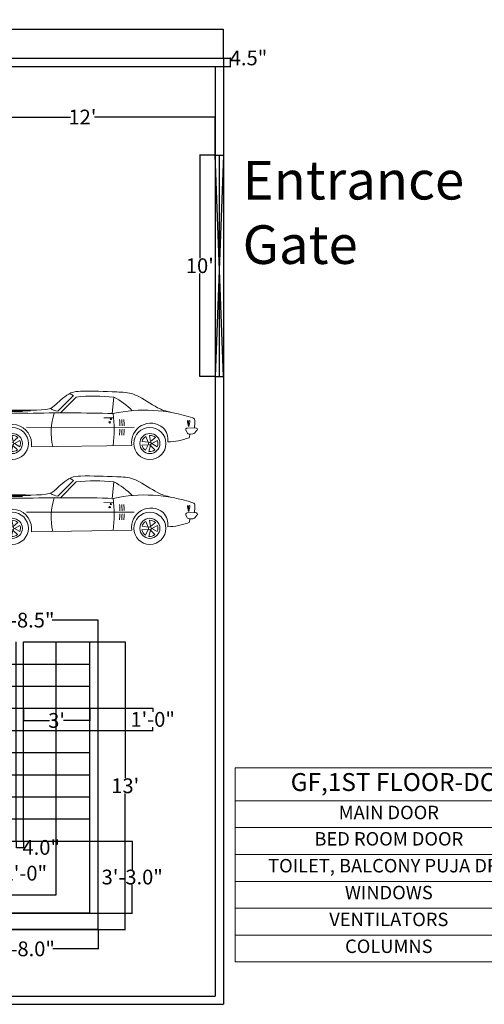
# Model space of a CAD drawing. Units: inches. Extents: x 20414 to 21627, y 49019 to 50314.
# Tile 9 of 10: x 20835 to 21087, y 49781 to 50314. Entities that reach past the tile are written whole.
import ezdxf

# ---------------------------------------------------------------- set-up
doc = ezdxf.new("R2010")
doc.units = ezdxf.units.IN
for name, color, linetype, lineweight in [('A-ANNO-DIMS', 7, 'Continuous', 18), ('A-ANNO-SCHD', 7, 'Continuous', 18), ('C-PROP', 6, 'Continuous', 25), ('C-SITE-GATE', 3, 'Continuous', 25), ('cars', 40, 'Continuous', 13), ('stairs', 4, 'Continuous', 25), ('text', 3, 'Continuous', 25), ('walls', 6, 'Continuous', 35)]:
    doc.layers.add(name, color=color, linetype=linetype, lineweight=lineweight)
doc.styles.get("Standard").update_dxf_attribs({"font": 'arial.ttf'})
doc.dimstyles.get("Standard").update_dxf_attribs({"dimtxt": 8, "dimasz": 0.18, "dimexe": 0.18, "dimexo": 0.0625, "dimgap": 0.09, "dimtad": 0, "dimtih": 1, "dimtoh": 1, "dimdec": 1, "dimzin": 0, "dimdsep": 46, "dimlunit": 3, "dimtxsty": 'Standard', "dimcen": 0.09, "dimadec": 0, "dimazin": 0, "dimtfac": 1, "dimtdec": 1, "dimtofl": 0, "dimtmove": 0, "dimatfit": 3, "dimfxl": 1, "dimtolj": 1, "dimtzin": 0, "dimarcsym": 0})

# ---------------------------------------------------------------- blocks, each defined once
blk = doc.blocks.new('*U25')
for p, q in [((1852, 1022), (2179, 1351)), ((1905, 986), (2237, 1320)), ((3032, 1318), (2995, 973)), ((1273, 1043), (872, 1041)), ((1099, 1012), (893, 1010)), ((897, 1028), (1273, 1032)), ((2822, 882), (3009, 880)), ((1185, 681), (3462, 680)), ((4581, 665), (4763, 671)), ((189, 502), (247, 503)), ((248, 455), (217, 455)), ((263, 487), (264, 471)), ((4554, 619), (4578, 571)), ((4639, 537), (4697, 540)), ((4742, 563), (4788, 619)), ((1292, 344), (1293, 267))]:
    blk.add_line(p, q)
for points in [[(897, 1014), (897, 1023, 0.269532), (893, 1030), (873, 1041, 0.575383), (867, 1037), (868, 1028, 0.269532), (872, 1022), (891, 1011, 0.575383)], [(724, 383), (854, 366), (804, 487, 0.199906)], [(880, 509), (903, 380), (1003, 465, 0.199906)], [(3628, 383), (3758, 366), (3709, 487, 0.199906)], [(3784, 509), (3808, 380), (3908, 465, 0.199906)], [(795, 196), (852, 314), (721, 305, 0.199906)], [(995, 206), (901, 297), (870, 170, 0.199906)], [(1048, 400), (932, 338), (1044, 269, 0.199906)], [(3700, 196), (3757, 314), (3626, 305, 0.199906)], [(3900, 206), (3805, 297), (3774, 170, 0.199906)], [(3952, 400), (3837, 338), (3948, 269, 0.199906)]]:
    blk.add_lwpolyline(points, format="xyb", close=True)
for points in [[(4612, 698), (4611, 811), (4584, 824)], [(4612, 698), (4611, 811), (4637, 824)], [(1293, 267), (3413, 300)]]:
    blk.add_lwpolyline(points)
for centre, radius in [((888, 339), 339), ((2944, 788), 15.7), ((3793, 339), 339), ((888, 339), 212), ((3793, 339), 212), ((888, 339), 31.7), ((3793, 339), 31.7)]:
    blk.add_circle(centre, radius)
for centre, radius, start, end in [((2911, 2669), 1508, 237.6103, 240.9785), ((2628, -2413), 3754, 83.8163, 95.9705), ((2426, 99), 1362, 43.2748, 63.5665), ((1861, 1282), 261, 230.424, 268.0085), ((3687, -2156), 3200, 71.5283, 102.1242), ((1071, -2828), 3808, 87.8393, 105.8096), ((522, -80), 1094, 98.5304, 116.112), ((2011, 765), 1938, 177.5773, 185.5205), ((2035, -34649), 35635, 88.423, 91.3179), ((3005, 572), 1299, 161.4307, 193.2363), ((652, 634), 2388, 351.8279, 8.1674), ((1159, 682), 2000, 0.852, 4.6556), ((1205, 682), 2000, 0.852, 4.6556), ((1250, 683), 2000, 0.852, 4.6556), ((4681, 819), 63.3, 357.932, 71.5283), ((888, 339), 404, 0.6373, 176.3412), ((1159, 682), 2000, 355.2644, 358.8633), ((1205, 682), 2000, 355.2644, 358.8633), ((1250, 683), 2000, 355.2644, 358.8633), ((3812, 365), 404, 49.2263, 189.1528), ((3795, 420), 377, 352.7285, 41.6613), ((4582, 633), 31.7, 91.939, 207.109), ((5493, 959), 919, 188.4683, 196.5315), ((3726, 939), 919, 344.7432, 352.8063), ((2960, 881), 1785, 353.1942, 357.932), ((4764, 639), 31.7, 320.1683, 91.939), ((248, 487), 15.8, 0.6373, 90.6373), ((248, 471), 15.8, 270.6373, 0.6373), ((4127, 1799), 1427, 271.6865, 290.2774), ((4635, 600), 63.3, 207.109, 273.4677), ((2902, 940), 1785, 344.3985, 346.9385), ((4693, 604), 63.3, 273.4677, 320.1683)]:
    blk.add_arc(centre, radius, start, end)
blk.add_ellipse((2969, 853), major_axis=(-16, -0.2), ratio=0.610043)
for points, knots in [([(289, 989), (459, 1021), (785, 1067), (1645, 1019), (1784, 1141), (2092, 1432), (2519, 1455), (2948, 1431), (3379, 1419), (3689, 1267), (3902, 1113), (4094, 1033), (4189, 1009), (4249, 994)], [18.629823, 18.629823, 18.629823, 18.629823, 19.527405, 20.700571, 21.107983, 21.608568, 21.92336, 23.151359, 23.716171, 23.908743, 24.77794, 24.943072, 25.187755, 25.187755, 25.187755, 25.187755]), ([(485, 365), (482, 361), (470, 351), (390, 381), (234, 354), (184, 564), (77, 575), (34, 600), (16, 684), (-24, 800), (39, 829), (38, 865), (38, 884), (38, 890), (39, 897), (40, 902)], [16.815853, 16.815853, 16.815853, 16.815853, 16.838212, 16.885395, 17.18439, 17.479846, 17.654423, 17.670693, 17.696923, 18.016358, 18.052739, 18.140805, 18.140805, 18.140805, 18.172382, 18.172382, 18.172382, 18.172382])]:
    blk.add_open_spline(points, degree=3, knots=knots)
blk = doc.blocks.new('*D37')
at = {"layer": 'A-ANNO-DIMS', "color": 0, "lineweight": -2, "transparency": 16777216}
for p, q in [((20877.55, 49977.01), (20892.4, 49977.01)), ((20892.22, 49976.83), (20892.22, 49903.18)), ((20892.22, 49821.19), (20892.22, 49894.83)), ((20877.55, 49821.01), (20892.4, 49821.01))]:
    blk.add_line(p, q, dxfattribs=at)
at = {"layer": 'A-ANNO-DIMS', "color": 0, "transparency": 16777216}
for points in [[(20892.19, 49976.83), (20892.25, 49976.83), (20892.22, 49977.01)], [(20892.19, 49821.19), (20892.25, 49821.19), (20892.22, 49821.01)]]:
    blk.add_solid(points, dxfattribs=at)
at = {"layer": 'Defpoints', "color": 0, "transparency": 16777216}
for p in [(20877.49, 49977.01), (20892.22, 49977.01), (20877.49, 49821.01)]:
    blk.add_point(p, dxfattribs=at)
at = {"layer": 'A-ANNO-DIMS', "color": 0, "transparency": 16777216, "insert": (20892.22, 49899.01), "char_height": 8, "attachment_point": 5}
blk.add_mtext("\\A1;13'", dxfattribs=at)
blk = doc.blocks.new('*D38')
at = {"layer": 'A-ANNO-DIMS', "color": 0, "lineweight": -2, "transparency": 16777216}
for p, q in [((20796.99, 49977.07), (20796.99, 49989.02)), ((20797.17, 49988.84), (20821.84, 49988.84)), ((20877.31, 49988.84), (20852.65, 49988.84)), ((20877.49, 49977.07), (20877.49, 49989.02))]:
    blk.add_line(p, q, dxfattribs=at)
at = {"layer": 'A-ANNO-DIMS', "color": 0, "transparency": 16777216}
for points in [[(20797.17, 49988.87), (20797.17, 49988.81), (20796.99, 49988.84)], [(20877.31, 49988.87), (20877.31, 49988.81), (20877.49, 49988.84)]]:
    blk.add_solid(points, dxfattribs=at)
at = {"layer": 'Defpoints', "color": 0, "transparency": 16777216}
for p in [(20877.49, 49988.84), (20796.99, 49977.01), (20877.49, 49977.01)]:
    blk.add_point(p, dxfattribs=at)
at = {"layer": 'A-ANNO-DIMS', "color": 0, "transparency": 16777216, "insert": (20837.24, 49988.84), "char_height": 8, "attachment_point": 5}
blk.add_mtext('\\A1;6\'-8.5"', dxfattribs=at)
blk = doc.blocks.new('*D39')
at = {"layer": 'A-ANNO-DIMS', "color": 0, "lineweight": -2, "transparency": 16777216}
for p, q in [((20873.05, 49869.01), (20896.18, 49869.01)), ((20896, 49868.83), (20896, 49853.68)), ((20896, 49830.19), (20896, 49845.33)), ((20873.05, 49830.01), (20896.18, 49830.01))]:
    blk.add_line(p, q, dxfattribs=at)
at = {"layer": 'A-ANNO-DIMS', "color": 0, "transparency": 16777216}
for points in [[(20895.97, 49868.83), (20896.03, 49868.83), (20896, 49869.01)], [(20895.97, 49830.19), (20896.03, 49830.19), (20896, 49830.01)]]:
    blk.add_solid(points, dxfattribs=at)
at = {"layer": 'Defpoints', "color": 0, "transparency": 16777216}
for p in [(20872.99, 49869.01), (20896, 49869.01), (20872.99, 49830.01)]:
    blk.add_point(p, dxfattribs=at)
at = {"layer": 'A-ANNO-DIMS', "color": 0, "transparency": 16777216, "insert": (20896, 49849.51), "char_height": 8, "attachment_point": 5}
blk.add_mtext('\\A1;3\'-3.0"', dxfattribs=at)
blk = doc.blocks.new('*D40')
at = {"layer": 'A-ANNO-DIMS', "color": 0, "lineweight": -2, "transparency": 16777216}
for p, q in [((20797.49, 49820.94), (20797.49, 49810.39)), ((20877.49, 49820.94), (20877.49, 49810.39)), ((20797.67, 49810.57), (20822.09, 49810.57)), ((20877.31, 49810.57), (20852.9, 49810.57))]:
    blk.add_line(p, q, dxfattribs=at)
at = {"layer": 'A-ANNO-DIMS', "color": 0, "transparency": 16777216}
for points in [[(20797.67, 49810.6), (20797.67, 49810.54), (20797.49, 49810.57)], [(20877.31, 49810.6), (20877.31, 49810.54), (20877.49, 49810.57)]]:
    blk.add_solid(points, dxfattribs=at)
at = {"layer": 'Defpoints', "color": 0, "transparency": 16777216}
for p in [(20797.49, 49821.01), (20877.49, 49821.01), (20877.49, 49810.57)]:
    blk.add_point(p, dxfattribs=at)
at = {"layer": 'A-ANNO-DIMS', "color": 0, "transparency": 16777216, "insert": (20837.49, 49810.57), "char_height": 8, "attachment_point": 5}
blk.add_mtext('\\A1;6\'-8.0"', dxfattribs=at)
blk = doc.blocks.new('*D42')
at = {"layer": 'A-ANNO-DIMS', "color": 0, "lineweight": -2, "transparency": 16777216}
for p, q in [((20832.99, 49868.94), (20832.99, 49865.42)), ((20836.99, 49868.94), (20836.99, 49865.42)), ((20833.17, 49865.6), (20836.81, 49865.6)), ((20836.99, 49865.6), (20837.17, 49865.6))]:
    blk.add_line(p, q, dxfattribs=at)
at = {"layer": 'A-ANNO-DIMS', "color": 0, "transparency": 16777216}
for points in [[(20833.17, 49865.63), (20833.17, 49865.57), (20832.99, 49865.6)], [(20836.81, 49865.63), (20836.81, 49865.57), (20836.99, 49865.6)]]:
    blk.add_solid(points, dxfattribs=at)
at = {"layer": 'Defpoints', "color": 0, "transparency": 16777216}
for p in [(20832.99, 49869.01), (20836.99, 49869.01), (20836.99, 49865.6)]:
    blk.add_point(p, dxfattribs=at)
at = {"layer": 'A-ANNO-DIMS', "color": 0, "transparency": 16777216, "insert": (20846.68, 49865.6), "char_height": 8, "attachment_point": 5}
blk.add_mtext('\\A1;4.0"', dxfattribs=at)
blk = doc.blocks.new('*D43')
at = {"layer": 'A-ANNO-DIMS', "color": 0, "lineweight": -2, "transparency": 16777216}
for p, q in [((20836.99, 49940.94), (20836.99, 49934.26)), ((20872.99, 49940.94), (20872.99, 49934.26)), ((20837.17, 49934.44), (20851.22, 49934.44)), ((20872.81, 49934.44), (20858.76, 49934.44))]:
    blk.add_line(p, q, dxfattribs=at)
at = {"layer": 'A-ANNO-DIMS', "color": 0, "transparency": 16777216}
for points in [[(20837.17, 49934.47), (20837.17, 49934.41), (20836.99, 49934.44)], [(20872.81, 49934.47), (20872.81, 49934.41), (20872.99, 49934.44)]]:
    blk.add_solid(points, dxfattribs=at)
at = {"layer": 'Defpoints', "color": 0, "transparency": 16777216}
for p in [(20836.99, 49941.01), (20872.99, 49941.01), (20872.99, 49934.44)]:
    blk.add_point(p, dxfattribs=at)
at = {"layer": 'A-ANNO-DIMS', "color": 0, "transparency": 16777216, "insert": (20854.99, 49934.44), "char_height": 8, "attachment_point": 5}
blk.add_mtext("\\A1;3'", dxfattribs=at)
blk = doc.blocks.new('*T57')
at = {"layer": 'A-ANNO-SCHD', "transparency": 16777216}
for p, q in [((0, 0), (411.04, 0)), ((0, 0), (0, -105.19)), ((411.04, 0), (411.04, -105.19)), ((0, -17.8), (411.04, -17.8)), ((166.47, -17.8), (166.47, -105.19)), ((205.52, -17.8), (205.52, -105.19)), ((308.28, -17.8), (308.28, -105.19)), ((0, -32.37), (411.04, -32.37)), ((0, -46.93), (411.04, -46.93)), ((0, -61.49), (411.04, -61.49)), ((0, -76.06), (411.04, -76.06)), ((0, -90.62), (411.04, -90.62)), ((0, -105.19), (411.04, -105.19))]:
    blk.add_line(p, q, dxfattribs=at)
at = {"layer": 'A-ANNO-SCHD', "color": 0, "transparency": 16777216}
for s, insert, char_height, width, attachment_point in [('GF,1ST FLOOR-DOORS,WINDOWS,COLUMNS SCHEDULES', (205.52, -8.9), 9.7096, 406.1845, 5), ('MAIN DOOR', (83.23, -25.08), 7.282, 161.6127, 5), ("4'*7'", (185.99, -25.08), 7.282, 34.1974, 5), ('2 NOS.', (256.9, -25.08), 7.282, 97.905, 5), ('BED ROOM DOOR', (83.23, -34.79), 7.2822, 161.6127, 2), ("3'*7'", (185.99, -34.79), 7.282, 34.1974, 2), ('5 NOS', (256.9, -34.79), 7.282, 97.905, 2), ('TOILET, BALCONY PUJA DRS', (83.23, -49.36), 7.2822, 161.6127, 2), ("2'6''*7'", (185.99, -49.36), 7.282, 34.1974, 2), ('7 NOS', (256.9, -49.36), 7.282, 97.905, 2), ('WINDOWS', (83.23, -63.92), 7.282, 161.6127, 2), ("3'*4'", (185.99, -63.92), 7.282, 34.1974, 2), ('16 NOS', (256.9, -63.92), 7.282, 97.905, 2), ('VENTILATORS', (83.23, -78.49), 7.2822, 161.6127, 2), ("2'*2'", (185.99, -78.49), 7.282, 34.1974, 2), ('5 NOS', (256.9, -78.49), 7.282, 97.905, 2), ('COLUMNS', (83.23, -93.05), 7.282, 161.6127, 2), ("9''*9''", (185.99, -93.05), 7.282, 34.1974, 2), ('12 NOS', (256.9, -93.05), 7.282, 97.905, 2)]:
    blk.add_mtext(s, dxfattribs=dict(at, insert=insert, char_height=char_height, width=width, attachment_point=attachment_point))
blk = doc.blocks.new('*D59')
at = {"layer": 'A-ANNO-DIMS', "color": 0, "lineweight": -2, "transparency": 16777216}
for p, q in [((20796.99, 50241.07), (20796.99, 50261.82)), ((20797.17, 50261.64), (20862.49, 50261.64)), ((20940.81, 50261.64), (20875.49, 50261.64)), ((20940.99, 50241.07), (20940.99, 50261.82))]:
    blk.add_line(p, q, dxfattribs=at)
at = {"layer": 'A-ANNO-DIMS', "color": 0, "transparency": 16777216}
for points in [[(20797.17, 50261.67), (20797.17, 50261.61), (20796.99, 50261.64)], [(20940.81, 50261.67), (20940.81, 50261.61), (20940.99, 50261.64)]]:
    blk.add_solid(points, dxfattribs=at)
at = {"layer": 'Defpoints', "color": 0, "transparency": 16777216}
for p in [(20940.99, 50261.64), (20796.99, 50241.01), (20940.99, 50241.01)]:
    blk.add_point(p, dxfattribs=at)
at = {"layer": 'A-ANNO-DIMS', "color": 0, "transparency": 16777216, "insert": (20868.99, 50261.64), "char_height": 8, "attachment_point": 5}
blk.add_mtext("\\A1;12'", dxfattribs=at)
blk = doc.blocks.new('*D61')
at = {"layer": 'A-ANNO-DIMS', "color": 0, "lineweight": -2, "transparency": 16777216}
for p, q in [((20468.49, 50293.57), (20468.49, 50309.35)), ((20468.67, 50309.17), (20688.5, 50309.17)), ((20945.31, 50309.17), (20725.48, 50309.17)), ((20945.49, 50293.57), (20945.49, 50309.35))]:
    blk.add_line(p, q, dxfattribs=at)
at = {"layer": 'A-ANNO-DIMS', "color": 0, "transparency": 16777216}
for points in [[(20468.67, 50309.2), (20468.67, 50309.14), (20468.49, 50309.17)], [(20945.31, 50309.2), (20945.31, 50309.14), (20945.49, 50309.17)]]:
    blk.add_solid(points, dxfattribs=at)
at = {"layer": 'Defpoints', "color": 0, "transparency": 16777216}
for p in [(20945.49, 50309.17), (20468.49, 50293.51), (20945.49, 50293.51)]:
    blk.add_point(p, dxfattribs=at)
at = {"layer": 'A-ANNO-DIMS', "color": 0, "transparency": 16777216, "insert": (20706.99, 50309.17), "char_height": 8, "attachment_point": 5}
blk.add_mtext('\\A1;39\'-9.0"', dxfattribs=at)
blk = doc.blocks.new('*D65')
at = {"layer": 'A-ANNO-DIMS', "color": 0, "lineweight": -2, "transparency": 16777216}
for p, q in [((20940.93, 50241.01), (20932.47, 50241.01)), ((20932.65, 50240.83), (20932.65, 50185.18)), ((20932.65, 50121.19), (20932.65, 50176.83)), ((20940.93, 50121.01), (20932.47, 50121.01))]:
    blk.add_line(p, q, dxfattribs=at)
at = {"layer": 'A-ANNO-DIMS', "color": 0, "transparency": 16777216}
for points in [[(20932.62, 50240.83), (20932.68, 50240.83), (20932.65, 50241.01)], [(20932.62, 50121.19), (20932.68, 50121.19), (20932.65, 50121.01)]]:
    blk.add_solid(points, dxfattribs=at)
at = {"layer": 'Defpoints', "color": 0, "transparency": 16777216}
for p in [(20932.65, 50241.01), (20940.99, 50241.01), (20940.99, 50121.01)]:
    blk.add_point(p, dxfattribs=at)
at = {"layer": 'A-ANNO-DIMS', "color": 0, "transparency": 16777216, "insert": (20932.65, 50181.01), "char_height": 8, "attachment_point": 5}
blk.add_mtext("\\A1;10'", dxfattribs=at)
blk = doc.blocks.new('*D69')
at = {"layer": 'A-ANNO-DIMS', "color": 0, "lineweight": -2, "transparency": 16777216}
for p, q in [((20941.05, 50293.51), (20949.54, 50293.51)), ((20949.36, 50293.51), (20949.36, 50293.69)), ((20949.36, 50293.69), (20949.54, 50293.69)), ((20949.36, 50289.19), (20949.36, 50293.33)), ((20941.05, 50289.01), (20949.54, 50289.01))]:
    blk.add_line(p, q, dxfattribs=at)
at = {"layer": 'A-ANNO-DIMS', "color": 0, "transparency": 16777216}
for points in [[(20949.33, 50293.33), (20949.39, 50293.33), (20949.36, 50293.51)], [(20949.33, 50289.19), (20949.39, 50289.19), (20949.36, 50289.01)]]:
    blk.add_solid(points, dxfattribs=at)
at = {"layer": 'Defpoints', "color": 0, "transparency": 16777216}
for p in [(20940.99, 50293.51), (20949.36, 50293.51), (20940.99, 50289.01)]:
    blk.add_point(p, dxfattribs=at)
at = {"layer": 'A-ANNO-DIMS', "color": 0, "transparency": 16777216, "insert": (20959.05, 50293.69), "char_height": 8, "attachment_point": 5}
blk.add_mtext('\\A1;4.5"', dxfattribs=at)
blk = doc.blocks.new('STAIR-RETURN-76IN')
for p, q in [((0, 0), (0, 156)), ((36, 48), (36, 156)), ((40, 48), (40, 156)), ((76, 9), (76, 156)), ((0, 144), (76, 144)), ((0, 132), (76, 132)), ((0, 120), (76, 120)), ((0, 108), (76, 108)), ((0, 96), (76, 96)), ((0, 84), (76, 84)), ((0, 72), (76, 72)), ((0, 60), (76, 60)), ((0, 48), (76, 48))]:
    blk.add_line(p, q)
blk.add_lwpolyline([(57.62, 156), (57.62, 18.61), (18.78, 18.61), (18.78, 138.01), (16.02, 133.61), (21.12, 133.61), (18.78, 138.01)])
blk = doc.blocks.new('*D118')
at = {"layer": 'A-ANNO-DIMS', "color": 0, "lineweight": -2, "transparency": 16777216}
for p, q in [((20733.71, 49848.07), (20733.71, 49851.79)), ((20733.89, 49851.61), (20757.53, 49851.61)), ((20757.71, 49848.07), (20757.71, 49851.79)), ((20757.71, 49851.61), (20757.89, 49851.61))]:
    blk.add_line(p, q, dxfattribs=at)
at = {"layer": 'A-ANNO-DIMS', "color": 0, "transparency": 16777216}
for points in [[(20733.89, 49851.64), (20733.89, 49851.58), (20733.71, 49851.61)], [(20757.53, 49851.64), (20757.53, 49851.58), (20757.71, 49851.61)]]:
    blk.add_solid(points, dxfattribs=at)
at = {"layer": 'Defpoints', "color": 0, "transparency": 16777216}
for p in [(20757.71, 49851.61), (20733.71, 49848.01), (20757.71, 49848.01)]:
    blk.add_point(p, dxfattribs=at)
at = {"layer": 'A-ANNO-DIMS', "color": 0, "transparency": 16777216, "insert": (20805.06, 49851.61), "char_height": 8, "attachment_point": 5}
blk.add_mtext('\\A1;MICROWAVE 2\'-0"', dxfattribs=at)
blk = doc.blocks.new('*D144')
at = {"layer": 'A-ANNO-DIMS', "color": 0, "lineweight": -2, "transparency": 16777216}
for p, q in [((20873.05, 49941.01), (20907.27, 49941.01)), ((20907.09, 49940.83), (20907.09, 49939.18)), ((20873.05, 49929.01), (20907.27, 49929.01)), ((20907.09, 49929.19), (20907.09, 49930.83))]:
    blk.add_line(p, q, dxfattribs=at)
at = {"layer": 'A-ANNO-DIMS', "color": 0, "transparency": 16777216}
for points in [[(20907.06, 49940.83), (20907.12, 49940.83), (20907.09, 49941.01)], [(20907.06, 49929.19), (20907.12, 49929.19), (20907.09, 49929.01)]]:
    blk.add_solid(points, dxfattribs=at)
at = {"layer": 'Defpoints', "color": 0, "transparency": 16777216}
for p in [(20872.99, 49941.01), (20872.99, 49929.01), (20907.09, 49929.01)]:
    blk.add_point(p, dxfattribs=at)
at = {"layer": 'A-ANNO-DIMS', "color": 0, "transparency": 16777216, "insert": (20907.09, 49935.01), "char_height": 8, "attachment_point": 5}
blk.add_mtext('\\A1;1\'-0"', dxfattribs=at)

msp = doc.modelspace()

# ---------------------------------------------------------------- linework, layer by layer
at = {"layer": 'C-PROP'}
for p, q in [((20468.49, 50293.51), (20945.49, 50293.51)), ((20945.49, 50293.51), (20945.49, 49780.51)), ((20472.99, 50289.01), (20940.99, 50289.01)), ((20940.99, 50289.01), (20940.99, 49785.01)), ((20796.99, 49785.01), (20940.99, 49785.01)), ((20468.49, 49780.51), (20945.49, 49780.51))]:
    msp.add_line(p, q, dxfattribs=at)
at = {"layer": 'C-SITE-GATE'}
for p, q in [((20940.99, 50241.01), (20945.49, 50241.01)), ((20945.49, 50121.01), (20940.99, 50241.01)), ((20945.49, 50241.01), (20940.99, 50121.01)), ((20943.24, 50121.01), (20943.24, 50241.01)), ((20940.99, 50121.01), (20945.49, 50121.01))]:
    msp.add_line(p, q, dxfattribs=at)
at = {"layer": 'stairs'}
for p in [(20836.99, 49977.01), (20877.49, 49821.01)]:
    msp.add_line(p, (20877.49, 49977.01), dxfattribs=at)
at = {"layer": 'walls'}
for p, q in [((20872.99, 49830.01), (20717.49, 49830.01)), ((20877.49, 49821.01), (20717.49, 49821.01))]:
    msp.add_line(p, q, dxfattribs=at)

# ---------------------------------------------------------------- block references
msp.add_blockref('*T57', (20951.88, 49908.67))
at = {"layer": 'cars', "xscale": 0.025666680406073, "yscale": 0.025666680406073, "zscale": 0.025666680406073}
for p in [(20808.22, 50075.9), (20808.22, 50029.9)]:
    msp.add_blockref('*U25', p, dxfattribs=at)
at = {"layer": 'stairs'}
msp.add_blockref('STAIR-RETURN-76IN', (20796.99, 49821.01), dxfattribs=at)

# ---------------------------------------------------------------- texts
at = {"layer": 'text', "insert": (20955.84, 50237.87), "char_height": 20.957, "attachment_point": 1}
msp.add_mtext_dynamic_manual_height_columns('Entrance Gate', width=93.1994, gutter_width=104.79, heights=[101.44], dxfattribs=at)

# ---------------------------------------------------------------- dimensions: what is measured, and where the dimension line sits
at = {"layer": 'A-ANNO-DIMS'}
for base, p1, p2, picture, middle in [((20945.49, 50309.17), (20468.49, 50293.51), (20945.49, 50293.51), '*D61', (20706.99, 50309.17)), ((20940.99, 50261.64), (20796.99, 50241.01), (20940.99, 50241.01), '*D59', (20868.99, 50261.64)), ((20877.49, 49988.84), (20796.99, 49977.01), (20877.49, 49977.01), '*D38', (20837.24, 49988.84)), ((20872.99, 49934.44), (20836.99, 49941.01), (20872.99, 49941.01), '*D43', (20854.99, 49934.44)), ((20836.99, 49865.6), (20832.99, 49869.01), (20836.99, 49869.01), '*D42', (20846.68, 49865.6)), ((20877.49, 49810.57), (20797.49, 49821.01), (20877.49, 49821.01), '*D40', (20837.49, 49810.57))]:
    dim = msp.add_linear_dim(base=base, p1=p1, p2=p2, dimstyle='Standard', override={"dimclrd": 0, "dimclre": 0, "dimclrt": 0}, dxfattribs=at)
    dim.commit()
    dim.dimension.update_dxf_attribs({"geometry": picture, "text_midpoint": middle})
for base, p1, p2, angle, override, picture, middle in [((20949.36, 50293.51), (20940.99, 50289.01), (20940.99, 50293.51), 90, {"dimclrd": 0, "dimclre": 0, "dimclrt": 0}, '*D69', (20959.05, 50293.69)), ((20932.65, 50241.01), (20940.99, 50121.01), (20940.99, 50241.01), 90, {"dimclrd": 0, "dimclre": 0, "dimclrt": 0}, '*D65', (20932.65, 50181.01)), ((20892.22, 49977.01), (20877.49, 49821.01), (20877.49, 49977.01), 90, {"dimclrd": 0, "dimclre": 0, "dimclrt": 0}, '*D37', (20892.22, 49899.01)), ((20907.09, 49929.01), (20872.99, 49941.01), (20872.99, 49929.01), 270, {"dimdec": 1, "dimlfac": 1, "dimrnd": 0, "dimzin": 1, "dimdsep": 46, "dimlunit": 4, "dimfrac": 2}, '*D144', (20907.09, 49935.01)), ((20896, 49869.01), (20872.99, 49830.01), (20872.99, 49869.01), 90, {"dimclrd": 0, "dimclre": 0, "dimclrt": 0}, '*D39', (20896, 49849.51))]:
    dim = msp.add_linear_dim(base=base, p1=p1, p2=p2, angle=angle, dimstyle='Standard', override=override, dxfattribs=at)
    dim.commit()
    dim.dimension.update_dxf_attribs({"geometry": picture, "text_midpoint": middle})
dim = msp.add_linear_dim(base=(20757.71, 49851.61), p1=(20733.71, 49848.01), p2=(20757.71, 49848.01), text='MICROWAVE <>', dimstyle='Standard', override={"dimdec": 1, "dimlfac": 1, "dimrnd": 0, "dimzin": 1, "dimdsep": 46, "dimlunit": 4, "dimfrac": 2}, dxfattribs=at)
dim.commit()
dim.dimension.update_dxf_attribs({"geometry": '*D118', "text_midpoint": (20805.06, 49851.61)})

doc.saveas('drawing.dxf')
